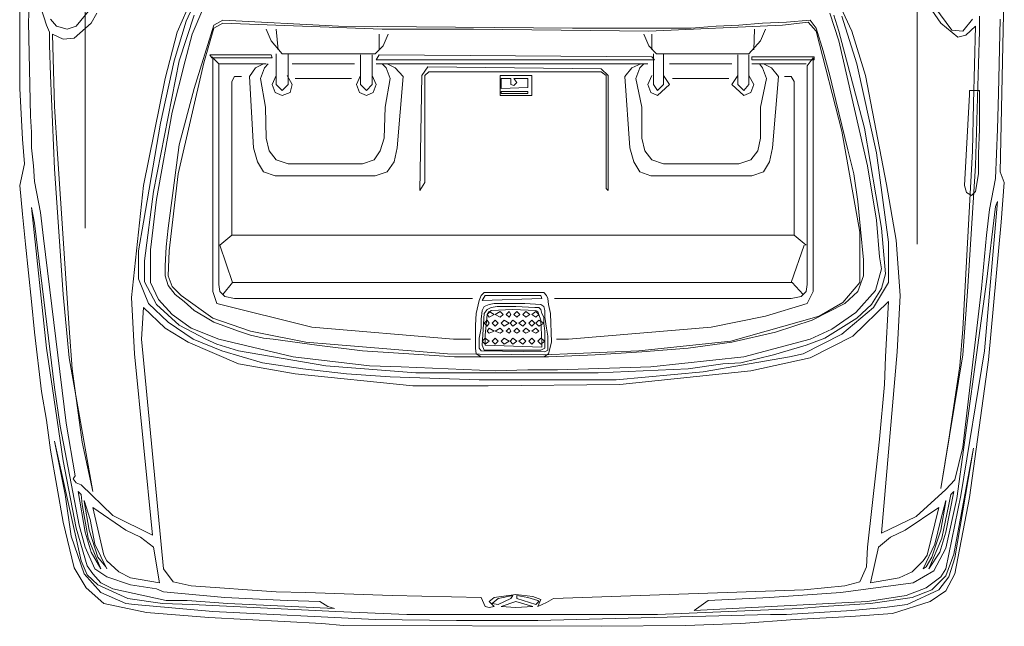
# Model space of a CAD drawing. Units: inches. Extents: x -36302355 to 648, y -221479757 to 75.
# Tile 5 of 37: x 185 to 224, y -531 to -507. Entities that reach past the tile are written whole.
import ezdxf

# ---------------------------------------------------------------- set-up
doc = ezdxf.new("R2010")
doc.units = ezdxf.units.IN
doc.header["$MEASUREMENT"] = 0
doc.layers.add('A-EQPM-VEHC', color=8, linetype='Continuous', lineweight=13)

msp = doc.modelspace()

# ---------------------------------------------------------------- linework, layer by layer
at = {"layer": 'A-EQPM-VEHC'}
for p, q in [((187.977, -500.428), (187.977, -514.82)), ((221.01, -500.979), (221.01, -515.45)), ((185.382, -502.395), (185.382, -509.277)), ((185.815, -504.204), (185.737, -506.642)), ((224.312, -512.579), (224.47, -504.794)), ((218.413, -506.996), (217.667, -505.383)), ((186.444, -506.759), (186.089, -505.659)), ((191.634, -507.035), (192.343, -505.422)), ((192.461, -505.58), (191.989, -506.603)), ((188.174, -506.131), (187.623, -506.799)), ((192.657, -506.131), (192.224, -507.114)), ((221.599, -506.17), (221.952, -506.682)), ((222.385, -506.956), (221.717, -506.052)), ((186.837, -506.799), (186.602, -506.524)), ((188.449, -506.287), (188.214, -506.682)), ((192.303, -506.366), (191.713, -508.175)), ((193.443, -506.563), (193.089, -506.759)), ((198.044, -506.799), (193.443, -506.563)), ((216.762, -506.563), (215.818, -506.642)), ((216.998, -506.878), (216.762, -506.563)), ((217.902, -507.389), (217.548, -506.287)), ((217.902, -506.996), (217.706, -506.366)), ((218.611, -508.293), (218.02, -506.406)), ((223.212, -506.524), (222.817, -506.996)), ((223.486, -506.996), (223.486, -506.406)), ((224.312, -506.524), (224.233, -509.474)), ((185.737, -506.642), (185.815, -510.377)), ((186.561, -507.035), (186.444, -506.759)), ((187.27, -506.917), (186.837, -506.799)), ((187.623, -506.799), (187.27, -506.917)), ((188.214, -506.682), (187.546, -507.271)), ((191.989, -506.603), (191.517, -508.175)), ((193.089, -506.759), (192.303, -509.277)), ((193.089, -506.878), (192.696, -508.254)), ((193.443, -506.682), (193.089, -506.878)), ((199.774, -506.917), (193.443, -506.682)), ((195.173, -506.917), (195.37, -507.389)), ((195.567, -506.917), (195.645, -507.743)), ((207.325, -506.878), (198.044, -506.799)), ((203.392, -506.917), (199.774, -506.917)), ((210.352, -506.996), (203.392, -506.917)), ((212.043, -506.878), (207.325, -506.878)), ((215.661, -506.759), (210.352, -506.996)), ((213.026, -506.799), (212.043, -506.878)), ((213.931, -506.759), (213.026, -506.799)), ((214.875, -506.682), (213.931, -506.759)), ((214.559, -506.917), (214.521, -507.743)), ((214.993, -506.917), (214.796, -507.389)), ((215.818, -506.642), (214.875, -506.682)), ((216.683, -506.642), (215.661, -506.759)), ((216.998, -506.996), (216.683, -506.642)), ((217.274, -507.782), (216.998, -506.878)), ((221.952, -506.682), (222.621, -507.231)), ((222.817, -506.996), (222.385, -506.956)), ((222.936, -507.154), (223.329, -506.799)), ((223.329, -506.799), (223.25, -509.867)), ((186.561, -507.547), (186.561, -507.035)), ((187.112, -507.31), (186.681, -507.114)), ((186.681, -507.114), (186.758, -509.984)), ((187.546, -507.271), (187.112, -507.31)), ((191.162, -508.884), (191.634, -507.035)), ((192.224, -507.114), (191.95, -508.175)), ((199.657, -507.114), (199.657, -507.743)), ((199.815, -507.586), (200.011, -507.114)), ((210.352, -507.586), (210.155, -507.114)), ((210.471, -507.114), (210.471, -507.743)), ((218.02, -510.967), (216.998, -506.996)), ((218.925, -510.849), (217.902, -506.996)), ((218.964, -508.765), (218.413, -506.996)), ((222.621, -507.231), (222.936, -507.154)), ((223.447, -508.293), (223.486, -506.996)), ((186.602, -508.765), (186.561, -507.547)), ((195.37, -507.389), (195.803, -507.9)), ((199.499, -507.9), (199.815, -507.586)), ((210.667, -507.9), (210.352, -507.586)), ((214.796, -507.389), (214.324, -507.9)), ((219.043, -512.344), (217.902, -507.389)), ((195.37, -507.94), (192.933, -507.94)), ((192.933, -507.94), (193.012, -508.058)), ((193.012, -508.019), (193.287, -508.293)), ((193.012, -508.058), (195.41, -508.058)), ((193.05, -508.058), (193.05, -517.338)), ((195.41, -508.058), (195.37, -507.94)), ((195.567, -509.119), (195.567, -507.9)), ((195.803, -507.9), (199.499, -507.9)), ((196.039, -507.9), (196.039, -509.119)), ((198.909, -509.119), (198.909, -507.94)), ((199.381, -507.94), (199.381, -509.119)), ((199.657, -507.94), (199.539, -508.136)), ((199.539, -508.136), (210.588, -508.136)), ((210.471, -508.019), (199.657, -507.94)), ((210.588, -508.136), (210.471, -508.019)), ((210.548, -509.119), (210.548, -507.9)), ((214.324, -507.9), (210.667, -507.9)), ((210.943, -507.9), (210.943, -509.119)), ((213.891, -509.119), (213.891, -507.94)), ((214.324, -507.94), (214.324, -509.119)), ((216.919, -508.019), (214.442, -508.019)), ((214.442, -508.019), (214.442, -508.136)), ((214.442, -508.136), (216.919, -508.136)), ((216.881, -508.058), (216.644, -508.372)), ((216.881, -508.058), (216.881, -517.338)), ((216.919, -508.136), (216.919, -508.019)), ((217.548, -508.765), (217.274, -507.782)), ((191.713, -508.175), (190.69, -513.366)), ((191.517, -508.175), (190.966, -510.653)), ((191.95, -508.175), (191.438, -510.219)), ((192.696, -508.254), (191.674, -512.658)), ((195.173, -508.293), (193.287, -508.293)), ((193.287, -508.293), (193.287, -517.063)), ((194.505, -508.805), (194.742, -508.451)), ((194.742, -508.451), (195.056, -508.293)), ((194.938, -508.884), (195.095, -508.451)), ((195.095, -508.451), (195.252, -508.293)), ((198.674, -508.293), (196.196, -508.293)), ((210.313, -508.293), (199.539, -508.293)), ((199.774, -508.293), (199.932, -508.451)), ((199.932, -508.451), (200.088, -508.884)), ((199.971, -508.293), (200.285, -508.451)), ((200.285, -508.451), (200.601, -508.805)), ((201.583, -508.412), (201.348, -508.765)), ((208.465, -508.489), (201.583, -508.412)), ((208.741, -508.765), (208.465, -508.489)), ((209.409, -508.805), (209.683, -508.451)), ((209.683, -508.451), (210.038, -508.293)), ((209.841, -508.884), (209.999, -508.451)), ((209.999, -508.451), (210.155, -508.293)), ((213.656, -508.293), (211.178, -508.293)), ((216.605, -508.293), (214.442, -508.293)), ((214.756, -508.293), (214.875, -508.451)), ((214.875, -508.451), (215.031, -508.884)), ((214.914, -508.293), (215.228, -508.451)), ((215.228, -508.451), (215.503, -508.805)), ((216.644, -508.372), (216.644, -517.063)), ((219.397, -511.832), (218.611, -508.293)), ((223.329, -512.344), (223.447, -508.293)), ((186.758, -512.462), (186.602, -508.765)), ((190.297, -513.13), (191.162, -508.884)), ((193.915, -508.805), (193.798, -509.002)), ((194.191, -508.805), (193.915, -508.805)), ((194.663, -511.635), (194.505, -508.805)), ((195.135, -510.023), (194.938, -508.884)), ((195.41, -509.119), (195.567, -508.765)), ((196, -508.765), (196.196, -509.119)), ((196.314, -508.884), (198.555, -508.884)), ((198.751, -509.119), (198.909, -508.765)), ((199.381, -508.765), (199.539, -509.119)), ((200.088, -508.884), (199.892, -510.023)), ((200.601, -508.805), (200.364, -511.635)), ((201.348, -508.765), (201.269, -513.327)), ((201.466, -508.765), (201.622, -508.608)), ((201.466, -513.013), (201.466, -508.765)), ((201.622, -508.608), (208.465, -508.608)), ((205.712, -508.765), (204.454, -508.765)), ((204.454, -508.765), (204.454, -509.552)), ((204.886, -508.884), (204.493, -508.884)), ((204.493, -508.884), (204.493, -509.277)), ((204.886, -509.119), (204.886, -508.884)), ((205.554, -508.884), (205.005, -508.884)), ((205.005, -508.884), (205.123, -509.04)), ((205.554, -509.237), (205.554, -508.884)), ((205.712, -509.552), (205.712, -508.765)), ((208.465, -508.608), (208.662, -508.765)), ((208.662, -508.765), (208.662, -513.248)), ((208.741, -513.327), (208.741, -508.765)), ((209.606, -511.635), (209.409, -508.805)), ((210.078, -510.023), (209.841, -508.884)), ((210.313, -509.119), (210.471, -508.765)), ((210.943, -508.765), (211.178, -509.119)), ((211.296, -508.884), (213.538, -508.884)), ((213.656, -509.119), (213.891, -508.765)), ((214.324, -508.765), (214.521, -509.119)), ((215.031, -508.884), (214.796, -510.023)), ((215.503, -508.805), (215.268, -511.635)), ((215.74, -508.805), (216.014, -508.805)), ((216.014, -508.805), (216.133, -509.002)), ((217.785, -509.749), (217.548, -508.765)), ((219.79, -513.09), (218.964, -508.765)), ((185.382, -509.277), (185.5, -511.283)), ((192.303, -509.277), (191.713, -511.518)), ((193.798, -509.002), (193.798, -515.096)), ((195.528, -509.433), (195.41, -509.119)), ((195.803, -509.354), (195.567, -509.119)), ((196.039, -509.119), (195.803, -509.354)), ((196.196, -509.119), (196.117, -509.433)), ((198.871, -509.433), (198.751, -509.119)), ((199.146, -509.354), (198.909, -509.119)), ((199.381, -509.119), (199.146, -509.354)), ((199.539, -509.119), (199.42, -509.433)), ((204.493, -509.277), (205.554, -509.237)), ((205.005, -509.158), (204.886, -509.119)), ((205.123, -509.04), (205.005, -509.158)), ((210.431, -509.433), (210.313, -509.119)), ((210.706, -509.354), (210.548, -509.119)), ((211.178, -509.119), (210.706, -509.552)), ((210.943, -509.119), (210.706, -509.354)), ((214.128, -509.552), (213.656, -509.119)), ((214.128, -509.354), (213.891, -509.119)), ((214.324, -509.119), (214.128, -509.354)), ((214.521, -509.119), (214.403, -509.433)), ((216.133, -509.002), (216.133, -515.096)), ((195.803, -509.552), (195.528, -509.433)), ((196.117, -509.433), (195.803, -509.552)), ((199.146, -509.552), (198.871, -509.433)), ((199.42, -509.433), (199.146, -509.552)), ((204.454, -509.552), (205.712, -509.552)), ((205.554, -509.395), (204.493, -509.395)), ((204.493, -509.395), (204.493, -509.474)), ((204.493, -509.474), (205.554, -509.474)), ((205.554, -509.474), (205.554, -509.395)), ((210.706, -509.552), (210.431, -509.433)), ((214.403, -509.433), (214.128, -509.552)), ((223.093, -509.512), (222.896, -513.13)), ((223.486, -509.354), (223.093, -509.354)), ((223.093, -509.354), (223.093, -509.512)), ((223.486, -510.888), (223.486, -509.354)), ((224.233, -509.474), (224.194, -510.888)), ((186.758, -509.984), (186.877, -511.872)), ((195.173, -511.242), (195.135, -510.023)), ((199.892, -510.023), (199.853, -511.242)), ((210.078, -511.242), (210.078, -510.023)), ((214.796, -510.023), (214.796, -511.242)), ((218.02, -510.732), (217.785, -509.749)), ((223.25, -509.867), (223.212, -511.753)), ((185.815, -510.377), (185.854, -511.007)), ((191.438, -510.219), (190.809, -513.681)), ((190.966, -510.653), (190.297, -514.585)), ((218.257, -511.714), (218.02, -510.732)), ((219.594, -514.82), (218.925, -510.849)), ((185.854, -511.007), (185.854, -511.635)), ((195.291, -511.753), (195.173, -511.242)), ((199.853, -511.242), (199.695, -511.753)), ((210.195, -511.753), (210.078, -511.242)), ((214.796, -511.242), (214.679, -511.753)), ((218.729, -514.978), (218.02, -510.967)), ((223.447, -511.872), (223.486, -510.888)), ((224.194, -510.888), (224.116, -512.855)), ((185.5, -511.283), (185.579, -512.265)), ((185.854, -511.635), (185.933, -512.344)), ((191.713, -511.518), (191.478, -513.327)), ((194.819, -512.186), (194.663, -511.635)), ((200.364, -511.635), (200.246, -512.186)), ((209.762, -512.186), (209.606, -511.635)), ((215.268, -511.635), (215.149, -512.186)), ((186.877, -511.872), (187.349, -518.793)), ((195.567, -512.107), (195.291, -511.753)), ((199.695, -511.753), (199.46, -512.107)), ((210.471, -512.107), (210.195, -511.753)), ((214.679, -511.753), (214.403, -512.107)), ((218.492, -512.658), (218.257, -511.714)), ((219.869, -515.371), (219.397, -511.832)), ((223.212, -511.753), (222.817, -518.831)), ((223.447, -512.658), (223.447, -511.872)), ((185.579, -512.265), (185.382, -513.13)), ((185.933, -512.344), (185.972, -512.973)), ((195.056, -512.579), (194.819, -512.186)), ((196.039, -512.265), (195.567, -512.107)), ((198.988, -512.265), (196.039, -512.265)), ((199.46, -512.107), (198.988, -512.265)), ((200.246, -512.186), (199.971, -512.579)), ((209.999, -512.579), (209.762, -512.186)), ((210.943, -512.265), (210.471, -512.107)), ((213.931, -512.265), (210.943, -512.265)), ((214.403, -512.107), (213.931, -512.265)), ((215.149, -512.186), (214.914, -512.579)), ((219.397, -514.506), (219.043, -512.344)), ((223.014, -517.338), (223.329, -512.344)), ((187.112, -517.456), (186.758, -512.462)), ((191.674, -512.658), (191.32, -515.726)), ((195.528, -512.737), (195.056, -512.579)), ((199.499, -512.737), (195.528, -512.737)), ((199.971, -512.579), (199.499, -512.737)), ((210.431, -512.737), (209.999, -512.579)), ((214.442, -512.737), (210.431, -512.737)), ((214.914, -512.579), (214.442, -512.737)), ((218.65, -513.759), (218.492, -512.658)), ((223.329, -513.366), (223.447, -512.658)), ((224.47, -513.013), (224.312, -512.579)), ((185.382, -513.13), (185.5, -514.271)), ((185.972, -512.973), (186.209, -514.192)), ((189.825, -517.573), (190.297, -513.13)), ((201.269, -513.327), (201.466, -513.013)), ((220.183, -515.292), (219.79, -513.09)), ((222.896, -513.13), (222.975, -513.406)), ((224.116, -512.855), (223.879, -514.074)), ((224.351, -514.585), (224.47, -513.013)), ((190.69, -513.366), (190.337, -516.119)), ((191.478, -513.327), (191.281, -514.82)), ((208.662, -513.248), (208.741, -513.327)), ((222.975, -513.406), (223.172, -513.523)), ((223.172, -513.523), (223.329, -513.366)), ((185.972, -514.624), (185.854, -513.995)), ((185.854, -513.995), (186.444, -519.579)), ((190.809, -513.681), (190.573, -515.685)), ((218.767, -514.861), (218.65, -513.759)), ((223.682, -519.697), (224.194, -513.759)), ((224.116, -513.955), (223.761, -516.945)), ((224.194, -513.759), (224.116, -513.955)), ((185.5, -514.271), (185.619, -515.45)), ((186.209, -514.192), (186.326, -515.215)), ((223.879, -514.074), (223.761, -515.096)), ((186.758, -521.151), (185.972, -514.624)), ((190.297, -514.585), (190.101, -515.726)), ((219.515, -515.961), (219.397, -514.506)), ((223.84, -520.051), (224.351, -514.585)), ((191.281, -514.82), (191.202, -515.568)), ((193.798, -515.096), (193.326, -515.489)), ((216.133, -515.096), (193.798, -515.096)), ((216.133, -515.096), (216.605, -515.489)), ((218.729, -516.984), (218.729, -514.978)), ((218.885, -516.08), (218.767, -514.861)), ((219.75, -516.629), (219.594, -514.82)), ((223.761, -515.096), (223.565, -517.219)), ((185.619, -515.45), (185.854, -517.731)), ((186.326, -515.215), (187.23, -522.567)), ((193.326, -515.489), (193.836, -516.984)), ((216.526, -515.489), (216.014, -516.984)), ((219.869, -516.984), (219.869, -515.371)), ((220.341, -517.494), (220.183, -515.292)), ((190.101, -515.726), (190.101, -516.826)), ((190.573, -515.685), (190.573, -516.984)), ((191.202, -515.568), (191.162, -516.315)), ((191.32, -515.726), (191.281, -516.708)), ((190.337, -516.119), (190.337, -516.945)), ((191.162, -516.315), (191.162, -516.708)), ((218.885, -516.708), (218.885, -516.08)), ((219.594, -516.433), (219.515, -515.961)), ((191.162, -516.708), (191.281, -517.101)), ((191.281, -516.708), (191.438, -517.142)), ((218.65, -517.338), (218.885, -516.708)), ((219.357, -517.298), (219.594, -516.433)), ((219.594, -517.219), (219.75, -516.629)), ((190.101, -516.826), (190.494, -517.81)), ((190.337, -516.945), (190.809, -517.849)), ((190.573, -516.984), (190.887, -517.652)), ((191.281, -517.101), (191.555, -517.456)), ((193.287, -517.063), (193.326, -517.338)), ((193.836, -516.984), (193.443, -517.456)), ((216.054, -516.984), (193.836, -516.984)), ((216.486, -517.456), (216.054, -516.984)), ((216.644, -517.063), (216.605, -517.338)), ((218.06, -517.77), (218.729, -516.984)), ((219.279, -517.966), (219.869, -516.984)), ((223.761, -516.945), (222.582, -525.556)), ((187.349, -519.972), (187.112, -517.456)), ((191.438, -517.142), (191.792, -517.494)), ((191.555, -517.456), (191.91, -517.731)), ((191.792, -517.494), (193.05, -518.4)), ((193.05, -517.338), (193.208, -517.81)), ((193.326, -517.338), (193.522, -517.535)), ((203.707, -517.494), (203.628, -517.691)), ((203.824, -517.377), (203.707, -517.494)), ((203.864, -517.494), (203.747, -517.691)), ((206.184, -517.377), (203.824, -517.377)), ((206.067, -517.494), (203.864, -517.494)), ((206.105, -517.614), (206.067, -517.494)), ((206.302, -517.494), (206.184, -517.377)), ((206.342, -517.614), (206.302, -517.494)), ((216.605, -517.338), (216.409, -517.535)), ((216.881, -517.338), (216.644, -517.81)), ((218.139, -517.81), (218.65, -517.338)), ((218.571, -518.163), (219.357, -517.298)), ((219.201, -517.849), (219.594, -517.219)), ((220.222, -519.737), (220.341, -517.494)), ((223.565, -517.219), (222.817, -523.511)), ((222.817, -519.854), (223.014, -517.338)), ((185.854, -517.731), (185.972, -518.951)), ((189.944, -519.816), (189.825, -517.573)), ((190.494, -517.81), (191.281, -518.556)), ((190.809, -517.849), (191.713, -518.675)), ((190.887, -517.652), (191.438, -518.242)), ((191.91, -517.731), (192.303, -518.084)), ((193.208, -517.81), (196.983, -518.753)), ((193.522, -517.535), (193.915, -517.614)), ((193.915, -517.614), (203.352, -517.614)), ((203.628, -517.691), (203.51, -518.203)), ((203.747, -517.691), (206.105, -517.614)), ((204.021, -517.849), (203.824, -517.928)), ((204.217, -517.81), (204.021, -517.849)), ((205.437, -517.81), (204.217, -517.81)), ((206.067, -517.849), (205.437, -517.81)), ((206.184, -517.928), (206.067, -517.849)), ((206.381, -517.849), (206.342, -517.614)), ((206.46, -518.203), (206.381, -517.849)), ((216.014, -517.614), (206.616, -517.614)), ((216.644, -517.81), (214.993, -518.321)), ((216.409, -517.535), (216.014, -517.614)), ((216.841, -518.479), (218.139, -517.81)), ((217.116, -518.321), (218.06, -517.77)), ((219.869, -517.731), (218.453, -519.107)), ((218.611, -518.4), (219.201, -517.849)), ((219.75, -519.933), (219.869, -517.731)), ((190.297, -517.966), (190.22, -519.225)), ((191.162, -518.793), (190.297, -517.966)), ((191.438, -518.242), (192.185, -518.793)), ((192.303, -518.084), (192.696, -518.321)), ((203.51, -518.203), (203.471, -518.675)), ((203.747, -518.084), (203.707, -518.438)), ((203.824, -517.928), (203.747, -518.084)), ((203.824, -518.203), (203.747, -519.461)), ((203.943, -518.045), (203.824, -518.203)), ((203.943, -518.242), (203.864, -519.068)), ((204.1, -517.966), (203.943, -518.045)), ((204.1, -518.084), (203.943, -518.242)), ((203.943, -518.242), (204.021, -518.124)), ((204.021, -518.359), (203.943, -518.242)), ((204.021, -518.124), (204.217, -518.242)), ((204.217, -518.242), (204.021, -518.359)), ((204.336, -517.928), (204.1, -517.966)), ((204.965, -518.045), (204.1, -518.084)), ((204.257, -518.242), (204.454, -518.124)), ((204.454, -518.359), (204.257, -518.242)), ((205.084, -517.928), (204.336, -517.928)), ((204.454, -518.124), (204.572, -518.242)), ((204.572, -518.242), (204.454, -518.359)), ((204.689, -518.242), (204.808, -518.124)), ((204.808, -518.359), (204.689, -518.242)), ((204.808, -518.124), (204.886, -518.242)), ((204.886, -518.242), (204.808, -518.359)), ((205.87, -518.084), (204.965, -518.045)), ((205.005, -518.242), (205.123, -518.124)), ((205.123, -518.359), (205.005, -518.242)), ((205.83, -517.966), (205.084, -517.928)), ((205.123, -518.124), (205.24, -518.242)), ((205.24, -518.242), (205.123, -518.359)), ((205.358, -518.242), (205.477, -518.124)), ((205.477, -518.359), (205.358, -518.242)), ((205.477, -518.124), (205.633, -518.242)), ((205.633, -518.242), (205.477, -518.359)), ((205.712, -518.242), (205.87, -518.124)), ((205.87, -518.359), (205.712, -518.242)), ((205.988, -517.966), (205.83, -517.966)), ((205.949, -518.124), (205.87, -518.084)), ((205.87, -518.124), (205.988, -518.242)), ((205.988, -518.242), (205.87, -518.359)), ((205.988, -518.242), (205.949, -518.124)), ((206.067, -518.045), (205.988, -517.966)), ((206.067, -518.479), (205.988, -518.242)), ((206.105, -518.203), (206.067, -518.045)), ((206.184, -518.359), (206.105, -518.203)), ((206.223, -518.084), (206.184, -517.928)), ((206.223, -518.359), (206.223, -518.084)), ((206.498, -519.344), (206.46, -518.203)), ((217.627, -518.831), (218.571, -518.163)), ((218.02, -519.028), (219.279, -517.966)), ((191.281, -518.556), (192.264, -519.225)), ((191.713, -518.675), (192.775, -519.225)), ((192.696, -518.321), (193.089, -518.556)), ((193.05, -518.4), (194.545, -518.91)), ((193.089, -518.556), (194.073, -518.91)), ((203.471, -518.675), (203.471, -519.579)), ((203.707, -518.438), (203.707, -518.793)), ((203.824, -518.596), (203.943, -518.479)), ((203.943, -518.714), (203.824, -518.596)), ((203.943, -518.479), (204.021, -518.596)), ((204.021, -518.596), (203.943, -518.714)), ((204.14, -518.596), (204.257, -518.479)), ((204.257, -518.714), (204.14, -518.596)), ((204.257, -518.479), (204.375, -518.596)), ((204.375, -518.596), (204.257, -518.714)), ((204.493, -518.596), (204.612, -518.479)), ((204.612, -518.714), (204.493, -518.596)), ((204.612, -518.479), (204.808, -518.596)), ((204.808, -518.596), (204.612, -518.714)), ((204.847, -518.596), (204.965, -518.479)), ((204.965, -518.714), (204.847, -518.596)), ((204.965, -518.479), (205.123, -518.596)), ((205.123, -518.596), (204.965, -518.714)), ((205.201, -518.596), (205.358, -518.479)), ((205.358, -518.714), (205.201, -518.596)), ((205.358, -518.479), (205.477, -518.596)), ((205.477, -518.596), (205.358, -518.714)), ((205.595, -518.596), (205.712, -518.479)), ((205.712, -518.714), (205.595, -518.596)), ((205.712, -518.479), (205.83, -518.596)), ((205.83, -518.596), (205.712, -518.714)), ((205.87, -518.596), (205.988, -518.479)), ((205.988, -518.714), (205.87, -518.596)), ((205.988, -518.479), (206.184, -518.596)), ((206.184, -518.596), (205.988, -518.714)), ((206.105, -519.344), (206.067, -518.479)), ((206.184, -518.596), (206.184, -518.359)), ((206.223, -518.91), (206.184, -518.596)), ((206.302, -518.793), (206.223, -518.359)), ((214.993, -518.321), (212.829, -518.753)), ((213.615, -519.303), (217.116, -518.321)), ((215.386, -518.951), (216.841, -518.479)), ((217.351, -519.186), (218.611, -518.4)), ((185.972, -518.951), (186.247, -521.309)), ((187.349, -518.793), (187.467, -520.405)), ((192.068, -519.344), (191.162, -518.793)), ((192.185, -518.793), (193.287, -519.225)), ((194.073, -518.91), (194.545, -519.068)), ((194.545, -518.91), (194.938, -518.989)), ((194.545, -519.068), (195.056, -519.186)), ((194.938, -518.989), (196.747, -519.344)), ((196.983, -518.753), (202.606, -519.225)), ((203.707, -518.793), (203.628, -519.186)), ((203.864, -519.068), (203.864, -519.461)), ((203.943, -518.91), (204.021, -518.793)), ((204.021, -518.989), (203.943, -518.91)), ((204.021, -518.793), (204.217, -518.91)), ((204.217, -518.91), (204.021, -518.989)), ((204.257, -518.91), (204.454, -518.793)), ((204.454, -518.989), (204.257, -518.91)), ((204.454, -518.793), (204.572, -518.91)), ((204.572, -518.91), (204.454, -518.989)), ((204.689, -518.91), (204.808, -518.793)), ((204.808, -518.989), (204.689, -518.91)), ((204.808, -518.793), (204.886, -518.91)), ((204.886, -518.91), (204.808, -518.989)), ((205.005, -518.91), (205.123, -518.793)), ((205.123, -518.989), (205.005, -518.91)), ((205.123, -518.793), (205.24, -518.91)), ((205.24, -518.91), (205.123, -518.989)), ((205.358, -518.91), (205.477, -518.793)), ((205.477, -518.989), (205.358, -518.91)), ((205.477, -518.793), (205.633, -518.91)), ((205.633, -518.91), (205.477, -518.989)), ((205.712, -518.91), (205.87, -518.793)), ((205.87, -518.989), (205.712, -518.91)), ((205.87, -518.793), (205.988, -518.91)), ((205.988, -518.91), (205.87, -518.989)), ((206.223, -519.579), (206.223, -518.91)), ((206.342, -519.107), (206.302, -518.793)), ((212.829, -518.753), (207.167, -519.225)), ((213.656, -519.344), (215.386, -518.951)), ((216.486, -519.816), (218.02, -519.028)), ((216.762, -519.225), (217.627, -518.831)), ((222.817, -518.831), (222.7, -520.286)), ((190.22, -519.225), (191.085, -528.347)), ((194.073, -520.209), (192.068, -519.344)), ((192.264, -519.225), (193.405, -519.697)), ((192.775, -519.225), (193.208, -519.421)), ((193.208, -519.421), (194.073, -519.697)), ((193.287, -519.225), (196.235, -519.933)), ((195.056, -519.186), (195.449, -519.225)), ((195.449, -519.225), (197.179, -519.461)), ((196.747, -519.344), (202.369, -519.816)), ((197.179, -519.461), (198.988, -519.697)), ((202.606, -519.225), (203.275, -519.225)), ((203.628, -519.186), (203.628, -519.579)), ((203.747, -519.303), (203.864, -519.186)), ((203.864, -519.421), (203.747, -519.303)), ((203.747, -519.461), (203.824, -519.658)), ((203.864, -519.186), (204.021, -519.303)), ((204.021, -519.303), (203.864, -519.421)), ((203.864, -519.461), (206.105, -519.54)), ((204.14, -519.303), (204.257, -519.186)), ((204.257, -519.421), (204.14, -519.303)), ((204.257, -519.186), (204.375, -519.303)), ((204.375, -519.303), (204.257, -519.421)), ((204.493, -519.303), (204.612, -519.186)), ((204.612, -519.421), (204.493, -519.303)), ((204.612, -519.186), (204.808, -519.303)), ((204.808, -519.303), (204.612, -519.421)), ((204.847, -519.303), (204.965, -519.186)), ((204.965, -519.421), (204.847, -519.303)), ((204.965, -519.186), (205.123, -519.303)), ((205.123, -519.303), (204.965, -519.421)), ((205.201, -519.303), (205.358, -519.186)), ((205.358, -519.421), (205.201, -519.303)), ((205.358, -519.186), (205.477, -519.303)), ((205.477, -519.303), (205.358, -519.421)), ((205.595, -519.303), (205.712, -519.186)), ((205.712, -519.421), (205.595, -519.303)), ((205.712, -519.186), (205.83, -519.303)), ((205.83, -519.303), (205.712, -519.421)), ((205.949, -519.303), (206.067, -519.186)), ((206.067, -519.421), (205.949, -519.303)), ((206.067, -519.186), (206.223, -519.303)), ((206.223, -519.303), (206.067, -519.421)), ((206.105, -519.54), (206.105, -519.344)), ((206.342, -519.658), (206.342, -519.107)), ((206.381, -519.816), (206.498, -519.344)), ((207.167, -519.225), (206.695, -519.225)), ((209.959, -519.697), (213.615, -519.303)), ((211.926, -519.579), (213.656, -519.344)), ((214.128, -519.933), (216.762, -519.225)), ((215.307, -519.854), (216.605, -519.461)), ((216.605, -519.461), (217.351, -519.186)), ((218.453, -519.107), (216.762, -519.972)), ((186.444, -519.579), (186.681, -521.191)), ((190.652, -527.012), (189.944, -519.816)), ((193.405, -519.697), (195.017, -520.169)), ((194.073, -519.697), (197.533, -520.286)), ((198.988, -519.697), (200.836, -519.816)), ((200.836, -519.816), (202.645, -519.933)), ((202.369, -519.816), (206.184, -519.854)), ((203.471, -519.579), (203.51, -519.816)), ((203.51, -519.816), (203.707, -519.933)), ((203.628, -519.579), (203.707, -519.697)), ((203.707, -519.697), (206.223, -519.737)), ((203.824, -519.658), (206.067, -519.658)), ((206.067, -519.658), (206.223, -519.579)), ((206.184, -519.854), (209.959, -519.697)), ((206.184, -519.933), (206.381, -519.816)), ((206.223, -519.737), (206.342, -519.658)), ((206.381, -519.933), (208.228, -519.854)), ((208.228, -519.854), (210.078, -519.737)), ((210.078, -519.737), (211.926, -519.579)), ((214.01, -520.169), (215.307, -519.854)), ((215.937, -519.933), (216.486, -519.816)), ((219.594, -526.933), (220.222, -519.737)), ((221.952, -525.162), (222.817, -519.854)), ((222.74, -525.438), (223.682, -519.697)), ((188.292, -525.282), (187.349, -519.972)), ((196.314, -520.602), (194.073, -520.209)), ((195.017, -520.169), (196.628, -520.405)), ((196.235, -519.933), (199.264, -520.286)), ((202.645, -519.933), (206.381, -519.933)), ((210.431, -520.326), (214.128, -519.933)), ((211.926, -520.405), (213.301, -520.209)), ((212.515, -520.523), (215.937, -519.933)), ((213.301, -520.209), (214.01, -520.169)), ((216.762, -519.972), (214.403, -520.483)), ((219.711, -521.034), (219.75, -519.933)), ((223.093, -525.517), (223.84, -520.051)), ((187.467, -520.405), (187.86, -523.315)), ((200.994, -521.074), (196.314, -520.602)), ((196.628, -520.405), (198.358, -520.602)), ((197.533, -520.286), (201.111, -520.562)), ((198.358, -520.602), (200.088, -520.719)), ((199.264, -520.286), (200.522, -520.326)), ((200.522, -520.326), (204.257, -520.483)), ((201.111, -520.562), (208.348, -520.562)), ((204.257, -520.483), (205.554, -520.444)), ((205.554, -520.444), (206.735, -520.444)), ((206.735, -520.444), (210.431, -520.326)), ((208.348, -520.562), (211.926, -520.405)), ((209.055, -520.837), (212.515, -520.523)), ((214.403, -520.483), (209.213, -521.034)), ((222.7, -520.286), (222.268, -523.197)), ((200.088, -520.719), (203.628, -520.837)), ((203.628, -520.837), (209.055, -520.837)), ((209.213, -521.034), (203.982, -521.074)), ((219.515, -523.197), (219.711, -521.034)), ((186.247, -521.309), (186.444, -522.45)), ((186.681, -521.191), (187.112, -524.062)), ((186.995, -522.685), (186.758, -521.151)), ((203.982, -521.074), (200.994, -521.074)), ((186.444, -522.45), (186.602, -523.629)), ((187.23, -522.567), (187.584, -524.652)), ((187.742, -526.617), (186.995, -522.685)), ((187.821, -528.033), (186.758, -523.276)), ((186.758, -523.276), (187.191, -525.399)), ((187.86, -523.315), (188.292, -525.282)), ((219.397, -524.297), (219.515, -523.197)), ((222.268, -523.197), (221.952, -525.162)), ((186.602, -523.629), (187.112, -526.5)), ((223.25, -523.55), (222.464, -527.758)), ((222.817, -523.511), (222.503, -524.81)), ((222.503, -527.916), (223.25, -523.55)), ((187.112, -524.062), (187.623, -526.736)), ((219.043, -527.482), (219.397, -524.297)), ((187.584, -524.652), (187.505, -524.769)), ((187.505, -524.769), (187.623, -524.927)), ((187.623, -524.927), (187.821, -525.006)), ((222.503, -524.81), (222.149, -525.203)), ((187.702, -525.282), (187.977, -526.893)), ((187.821, -525.399), (187.702, -525.282)), ((187.821, -525.006), (189.079, -526.224)), ((222.149, -525.203), (220.969, -526.264)), ((222.464, -525.282), (222.149, -526.893)), ((222.345, -525.399), (222.464, -525.282)), ((187.191, -525.399), (187.426, -527.05)), ((187.86, -525.792), (187.821, -525.399)), ((188.174, -526.382), (187.939, -525.634)), ((187.939, -525.634), (187.939, -525.675)), ((187.939, -525.675), (188.135, -526.815)), ((221.952, -526.382), (222.149, -525.634)), ((222.149, -525.675), (221.952, -526.815)), ((222.149, -528.347), (222.74, -525.438)), ((222.582, -525.556), (222.149, -527.522)), ((222.149, -525.634), (222.149, -525.675)), ((222.268, -525.792), (222.345, -525.399)), ((222.503, -528.545), (223.093, -525.517)), ((188.095, -527.129), (187.86, -525.792)), ((189.59, -526.815), (188.292, -525.91)), ((188.292, -525.91), (188.725, -527.798)), ((220.538, -526.815), (221.875, -525.91)), ((221.875, -525.91), (221.403, -527.798)), ((221.992, -527.129), (222.268, -525.792)), ((187.112, -526.5), (187.546, -528.309)), ((188.37, -527.365), (188.174, -526.382)), ((189.079, -526.224), (190.652, -527.012)), ((220.969, -526.264), (219.594, -526.933)), ((221.717, -527.365), (221.952, -526.382)), ((187.623, -526.736), (188.056, -528.23)), ((187.977, -527.482), (187.742, -526.617)), ((187.977, -526.893), (188.214, -527.68)), ((188.135, -526.815), (188.488, -527.877)), ((190.18, -527.089), (189.59, -526.815)), ((219.946, -527.089), (220.538, -526.815)), ((221.952, -526.815), (221.599, -527.877)), ((222.149, -526.893), (221.913, -527.68)), ((187.426, -527.05), (187.939, -528.545)), ((188.607, -528.347), (188.095, -527.129)), ((190.69, -527.482), (190.18, -527.089)), ((219.476, -527.482), (219.946, -527.089)), ((221.48, -528.347), (221.992, -527.129)), ((188.37, -528.347), (187.977, -527.482)), ((188.214, -527.68), (188.607, -528.347)), ((188.842, -528.347), (188.37, -527.365)), ((190.927, -528.898), (190.69, -527.482)), ((219.004, -528.27), (219.043, -527.482)), ((219.16, -528.898), (219.476, -527.482)), ((221.245, -528.347), (221.717, -527.365)), ((221.913, -527.68), (221.48, -528.347)), ((222.149, -527.522), (221.678, -528.426)), ((188.056, -528.584), (187.821, -528.033)), ((188.488, -527.877), (188.804, -528.27)), ((188.725, -527.798), (188.842, -528.033)), ((188.842, -528.033), (189.314, -528.466)), ((221.245, -528.033), (220.813, -528.466)), ((221.403, -527.798), (221.245, -528.033)), ((221.599, -527.877), (221.362, -528.27)), ((222.464, -527.758), (222.149, -528.623)), ((222.268, -528.663), (222.503, -527.916)), ((187.546, -528.309), (188.018, -529.095)), ((188.056, -528.23), (188.292, -528.545)), ((188.842, -528.663), (188.37, -528.347)), ((188.804, -528.27), (188.842, -528.347)), ((189.314, -528.466), (189.786, -528.702)), ((191.085, -528.347), (191.478, -528.86)), ((218.729, -528.86), (219.004, -528.27)), ((220.813, -528.466), (220.301, -528.702)), ((221.678, -528.426), (220.852, -528.898)), ((221.362, -528.27), (221.245, -528.347)), ((221.952, -528.663), (222.149, -528.347)), ((187.939, -528.545), (188.607, -529.291)), ((188.488, -528.977), (188.056, -528.584)), ((188.292, -528.545), (188.607, -528.898)), ((189.786, -528.977), (188.842, -528.663)), ((189.786, -528.702), (190.927, -528.898)), ((220.301, -528.702), (219.16, -528.898)), ((221.362, -529.095), (221.952, -528.663)), ((222.149, -528.623), (221.599, -529.174)), ((221.875, -529.174), (222.268, -528.663)), ((222.149, -529.214), (222.503, -528.545)), ((188.018, -529.095), (188.725, -529.725)), ((189.669, -529.528), (188.488, -528.977)), ((188.607, -528.898), (189.079, -529.135)), ((189.079, -529.135), (191.202, -529.607)), ((190.809, -529.135), (189.786, -528.977)), ((191.085, -529.253), (190.809, -529.135)), ((191.478, -528.86), (192.185, -529.016)), ((192.185, -529.016), (193.326, -529.095)), ((193.326, -529.095), (194.426, -529.174)), ((194.426, -529.174), (195.567, -529.253)), ((206.577, -529.528), (216.526, -529.174)), ((216.526, -529.174), (218.139, -529.016)), ((220.852, -528.898), (217.981, -529.291)), ((218.139, -529.016), (218.729, -528.86)), ((220.576, -529.41), (221.362, -529.095)), ((220.615, -529.763), (221.875, -529.174)), ((221.599, -529.174), (220.813, -529.488)), ((221.52, -529.646), (222.149, -529.214)), ((188.607, -529.291), (189.59, -529.725)), ((191.045, -529.725), (189.669, -529.528)), ((193.522, -529.488), (191.085, -529.253)), ((191.202, -529.607), (192.027, -529.607)), ((192.027, -529.607), (193.64, -529.725)), ((196, -529.607), (193.522, -529.488)), ((195.567, -529.253), (196.747, -529.291)), ((197.297, -529.646), (196, -529.607)), ((196.747, -529.291), (200.167, -529.41)), ((200.167, -529.41), (203.707, -529.488)), ((203.707, -529.488), (203.864, -529.842)), ((204.021, -529.646), (204.217, -529.488)), ((204.375, -529.528), (204.14, -529.725)), ((204.217, -529.488), (205.084, -529.37)), ((204.965, -529.41), (204.375, -529.528)), ((204.375, -529.763), (204.886, -529.528)), ((204.886, -529.528), (204.965, -529.41)), ((205.084, -529.37), (205.751, -529.449)), ((205.554, -529.488), (205.123, -529.41)), ((205.123, -529.41), (205.123, -529.528)), ((205.123, -529.528), (205.87, -529.763)), ((205.949, -529.607), (205.554, -529.488)), ((205.751, -529.449), (206.067, -529.567)), ((206.067, -529.567), (205.949, -529.842)), ((205.988, -529.646), (205.949, -529.607)), ((206.302, -529.684), (206.577, -529.528)), ((212.712, -529.607), (212.161, -530)), ((215.149, -529.488), (212.712, -529.607)), ((217.981, -529.291), (215.149, -529.488)), ((219.043, -529.646), (220.576, -529.41)), ((220.813, -529.488), (219.16, -529.725)), ((188.725, -529.725), (190.416, -530.079)), ((189.59, -529.725), (189.944, -529.763)), ((189.944, -529.763), (193.05, -530.039)), ((192.224, -529.763), (191.045, -529.725)), ((197.927, -530.039), (192.224, -529.763)), ((193.64, -529.725), (197.886, -529.921)), ((197.612, -529.842), (197.297, -529.646)), ((197.886, -529.921), (197.612, -529.842)), ((203.864, -529.842), (204.021, -529.881)), ((204.217, -529.842), (204.021, -529.646)), ((204.021, -529.881), (204.217, -529.842)), ((204.14, -529.725), (204.375, -529.763)), ((205.084, -529.646), (204.493, -529.842)), ((204.493, -529.842), (205.084, -529.881)), ((205.751, -529.842), (205.084, -529.646)), ((205.084, -529.881), (205.751, -529.842)), ((205.87, -529.763), (205.988, -529.646)), ((205.949, -529.842), (206.302, -529.684)), ((212.161, -530), (219.043, -529.646)), ((216.369, -529.921), (213.538, -530.039)), ((215.818, -530.156), (218.413, -530)), ((217.274, -529.842), (216.369, -529.921)), ((219.16, -529.725), (217.274, -529.842)), ((218.413, -530), (219.711, -529.881)), ((219.711, -529.881), (220.615, -529.763)), ((220.025, -530.118), (221.52, -529.646)), ((190.416, -530.079), (192.892, -530.276)), ((192.892, -530.276), (197.376, -530.511)), ((193.05, -530.039), (199.499, -530.353)), ((200.757, -530.156), (197.927, -530.039)), ((199.499, -530.353), (202.724, -530.393)), ((210.706, -530.156), (200.757, -530.156)), ((202.724, -530.393), (205.949, -530.393)), ((205.949, -530.393), (215.189, -530.156)), ((213.538, -530.039), (210.706, -530.156)), ((214.01, -530.511), (216.172, -530.353)), ((215.189, -530.156), (215.818, -530.156)), ((216.172, -530.353), (218.374, -530.235)), ((218.374, -530.235), (220.025, -530.118)), ((197.376, -530.511), (198.241, -530.59)), ((198.241, -530.59), (208.465, -530.628)), ((208.465, -530.628), (211.808, -530.59)), ((211.808, -530.59), (214.01, -530.511))]:
    msp.add_line(p, q, dxfattribs=at)

doc.saveas('drawing.dxf')
